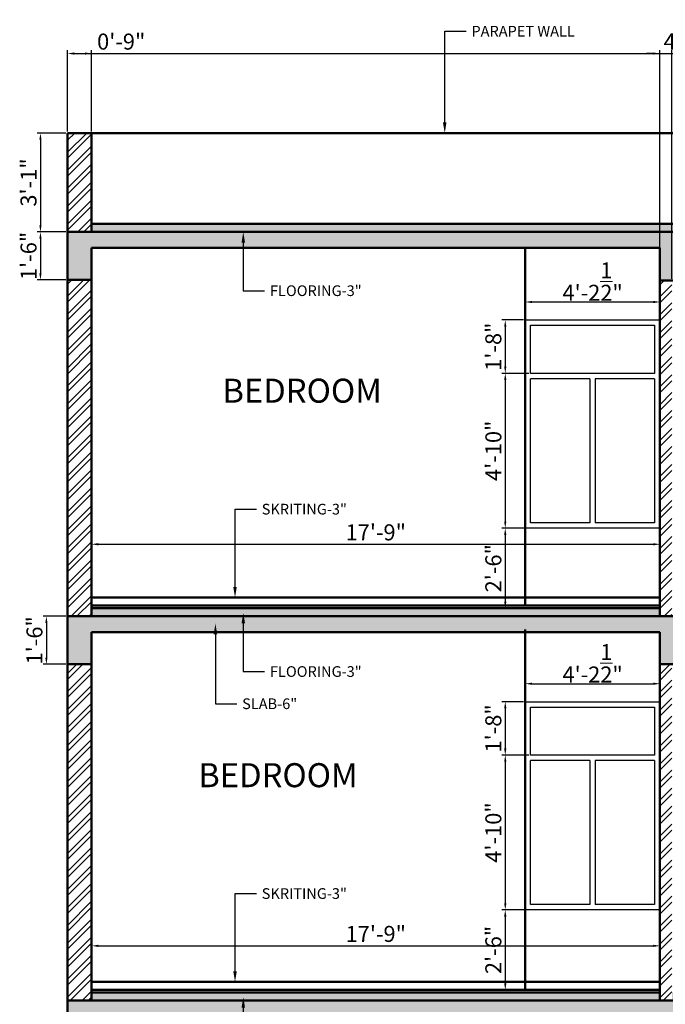
# Model space of a CAD drawing. Units: inches. Extents: x 1615 to 2231, y 1931 to 2519.
# Tile 2 of 6: x 1650 to 1892, y 2150 to 2519. Entities that reach past the tile are written whole.
import ezdxf
from ezdxf import colors
from ezdxf.entities.mleader import LeaderData, LeaderLine
from ezdxf.math import Vec2, Vec3

# ---------------------------------------------------------------- set-up
doc = ezdxf.new("R2010")
doc.units = ezdxf.units.IN
for name, color, linetype, lineweight in [('A-ANNO-DIMS', 2, 'Continuous', 18), ('A-ANNO-NOTE', 3, 'Continuous', 18), ('A-AREA-IDEN', 7, 'Continuous', 25), ('A-GLAZ', 4, 'Continuous', 25), ('A-SECT', 7, 'Continuous', 50), ('A-WALL-PATT', 8, 'Continuous', 13)]:
    doc.layers.add(name, color=color, linetype=linetype, lineweight=lineweight)
doc.styles.get("Standard").update_dxf_attribs({"font": 'arial.ttf'})
doc.dimstyles.new('ISO-25', dxfattribs={"dimtxt": 6, "dimasz": 2.5, "dimexe": 1.25, "dimexo": 0.625, "dimtad": 1, "dimdec": 1, "dimlunit": 4, "dimtxsty": 'Standard', "dimcen": 2.5, "dimadec": 0, "dimazin": 0, "dimtfac": 1, "dimtdec": 1, "dimtmove": 0, "dimatfit": 3, "dimfxl": 1, "dimarcsym": 0})

# ---------------------------------------------------------------- blocks, each defined once
blk = doc.blocks.new('*D2')
at = {"layer": 'A-ANNO-DIMS', "color": 0, "lineweight": -2, "transparency": 16777216}
for p, q in [((1667.24, 2476.53), (1656.46, 2476.53)), ((1657.71, 2474.03), (1657.71, 2442.03)), ((1667.24, 2439.53), (1656.46, 2439.53))]:
    blk.add_line(p, q, dxfattribs=at)
at = {"layer": 'A-ANNO-DIMS', "color": 0, "lineweight": 100, "transparency": 16777216}
for points in [[(1657.29, 2474.03), (1658.12, 2474.03), (1657.71, 2476.53)], [(1657.29, 2442.03), (1658.12, 2442.03), (1657.71, 2439.53)]]:
    blk.add_solid(points, dxfattribs=at)
at = {"layer": 'Defpoints', "color": 0, "lineweight": 100, "transparency": 16777216}
for p in [(1667.87, 2476.53), (1657.71, 2439.53), (1667.87, 2439.53)]:
    blk.add_point(p, dxfattribs=at)
at = {"layer": 'A-ANNO-DIMS', "color": 0, "transparency": 16777216, "insert": (1654.02, 2458.03), "char_height": 6, "attachment_point": 5, "rotation": 90}
blk.add_mtext('3\'-1"', dxfattribs=at)
blk = doc.blocks.new('*D3')
at = {"layer": 'A-ANNO-DIMS', "color": 0, "lineweight": -2, "transparency": 16777216}
for p, q in [((1667.24, 2439.53), (1656.46, 2439.53)), ((1657.71, 2437.03), (1657.71, 2424.03)), ((1667.24, 2421.53), (1656.46, 2421.53))]:
    blk.add_line(p, q, dxfattribs=at)
at = {"layer": 'A-ANNO-DIMS', "color": 0, "lineweight": 100, "transparency": 16777216}
for points in [[(1657.29, 2437.03), (1658.12, 2437.03), (1657.71, 2439.53)], [(1657.29, 2424.03), (1658.12, 2424.03), (1657.71, 2421.53)]]:
    blk.add_solid(points, dxfattribs=at)
at = {"layer": 'Defpoints', "color": 0, "lineweight": 100, "transparency": 16777216}
for p in [(1667.87, 2439.53), (1657.71, 2421.53), (1667.87, 2421.53)]:
    blk.add_point(p, dxfattribs=at)
at = {"layer": 'A-ANNO-DIMS', "color": 0, "transparency": 16777216, "insert": (1654.02, 2430.53), "char_height": 6, "attachment_point": 5, "rotation": 90}
blk.add_mtext('1\'-6"', dxfattribs=at)
blk = doc.blocks.new('*D4')
at = {"layer": 'A-ANNO-DIMS', "color": 0, "lineweight": -2, "transparency": 16777216}
for p, q in [((1667.24, 2295.53), (1658.68, 2295.53)), ((1659.93, 2293.03), (1659.93, 2280.03)), ((1667.24, 2277.53), (1658.68, 2277.53))]:
    blk.add_line(p, q, dxfattribs=at)
at = {"layer": 'A-ANNO-DIMS', "color": 0, "lineweight": 100, "transparency": 16777216}
for points in [[(1659.51, 2293.03), (1660.35, 2293.03), (1659.93, 2295.53)], [(1659.51, 2280.03), (1660.35, 2280.03), (1659.93, 2277.53)]]:
    blk.add_solid(points, dxfattribs=at)
at = {"layer": 'Defpoints', "color": 0, "lineweight": 100, "transparency": 16777216}
for p in [(1667.87, 2295.53), (1659.93, 2277.53), (1667.87, 2277.53)]:
    blk.add_point(p, dxfattribs=at)
at = {"layer": 'A-ANNO-DIMS', "color": 0, "transparency": 16777216, "insert": (1656.24, 2286.53), "char_height": 6, "attachment_point": 5, "rotation": 90}
blk.add_mtext('1\'-6"', dxfattribs=at)
blk = doc.blocks.new('*D33')
at = {"layer": 'A-ANNO-DIMS', "color": 0, "lineweight": -2, "transparency": 16777216}
for p, q in [((1839.37, 2264.15), (1839.37, 2271.52)), ((1841.87, 2270.27), (1887.37, 2270.27)), ((1889.87, 2264.15), (1889.87, 2271.52))]:
    blk.add_line(p, q, dxfattribs=at)
at = {"layer": 'A-ANNO-DIMS', "color": 0, "lineweight": 100, "transparency": 16777216}
for points in [[(1841.87, 2270.68), (1841.87, 2269.85), (1839.37, 2270.27)], [(1887.37, 2270.68), (1887.37, 2269.85), (1889.87, 2270.27)]]:
    blk.add_solid(points, dxfattribs=at)
at = {"layer": 'Defpoints', "color": 0, "lineweight": 100, "transparency": 16777216}
for p in [(1889.87, 2270.27), (1839.37, 2263.53), (1889.87, 2263.53)]:
    blk.add_point(p, dxfattribs=at)
at = {"layer": 'A-ANNO-DIMS', "color": 0, "transparency": 16777216, "insert": (1864.62, 2277.92), "char_height": 6, "attachment_point": 5}
blk.add_mtext('4\'-2{\\H1x;\\S1/2;}"', dxfattribs=at)
blk = doc.blocks.new('*D34')
at = {"layer": 'A-ANNO-DIMS', "color": 0, "lineweight": -2, "transparency": 16777216}
for p, q in [((1838.74, 2263.53), (1830.64, 2263.53)), ((1831.89, 2261.03), (1831.89, 2246.03)), ((1840.74, 2243.53), (1830.64, 2243.53))]:
    blk.add_line(p, q, dxfattribs=at)
at = {"layer": 'A-ANNO-DIMS', "color": 0, "lineweight": 100, "transparency": 16777216}
for points in [[(1831.47, 2261.03), (1832.31, 2261.03), (1831.89, 2263.53)], [(1831.47, 2246.03), (1832.31, 2246.03), (1831.89, 2243.53)]]:
    blk.add_solid(points, dxfattribs=at)
at = {"layer": 'Defpoints', "color": 0, "lineweight": 100, "transparency": 16777216}
for p in [(1839.37, 2263.53), (1831.89, 2243.53), (1841.37, 2243.53)]:
    blk.add_point(p, dxfattribs=at)
at = {"layer": 'A-ANNO-DIMS', "color": 0, "transparency": 16777216, "insert": (1828.2, 2253.53), "char_height": 6, "attachment_point": 5, "rotation": 90}
blk.add_mtext('1\'-8"', dxfattribs=at)
blk = doc.blocks.new('*D35')
at = {"layer": 'A-ANNO-DIMS', "color": 0, "lineweight": -2, "transparency": 16777216}
for p, q in [((1840.74, 2243.53), (1830.64, 2243.53)), ((1831.89, 2241.03), (1831.89, 2188.03)), ((1840.74, 2185.53), (1830.64, 2185.53))]:
    blk.add_line(p, q, dxfattribs=at)
at = {"layer": 'A-ANNO-DIMS', "color": 0, "lineweight": 100, "transparency": 16777216}
for points in [[(1831.47, 2241.03), (1832.31, 2241.03), (1831.89, 2243.53)], [(1831.47, 2188.03), (1832.31, 2188.03), (1831.89, 2185.53)]]:
    blk.add_solid(points, dxfattribs=at)
at = {"layer": 'Defpoints', "color": 0, "lineweight": 100, "transparency": 16777216}
for p in [(1841.37, 2243.53), (1831.89, 2185.53), (1841.37, 2185.53)]:
    blk.add_point(p, dxfattribs=at)
at = {"layer": 'A-ANNO-DIMS', "color": 0, "transparency": 16777216, "insert": (1828.2, 2214.53), "char_height": 6, "attachment_point": 5, "rotation": 90}
blk.add_mtext('4\'-10"', dxfattribs=at)
blk = doc.blocks.new('*D36')
at = {"layer": 'A-ANNO-DIMS', "color": 0, "lineweight": -2, "transparency": 16777216}
for p, q in [((1838.74, 2185.53), (1830.64, 2185.53)), ((1831.89, 2183.03), (1831.89, 2158.03)), ((1838.74, 2155.53), (1830.64, 2155.53))]:
    blk.add_line(p, q, dxfattribs=at)
at = {"layer": 'A-ANNO-DIMS', "color": 0, "lineweight": 100, "transparency": 16777216}
for points in [[(1831.47, 2183.03), (1832.31, 2183.03), (1831.89, 2185.53)], [(1831.47, 2158.03), (1832.31, 2158.03), (1831.89, 2155.53)]]:
    blk.add_solid(points, dxfattribs=at)
at = {"layer": 'Defpoints', "color": 0, "lineweight": 100, "transparency": 16777216}
for p in [(1839.37, 2185.53), (1831.89, 2155.53), (1839.37, 2155.53)]:
    blk.add_point(p, dxfattribs=at)
at = {"layer": 'A-ANNO-DIMS', "color": 0, "transparency": 16777216, "insert": (1828.2, 2170.53), "char_height": 6, "attachment_point": 5, "rotation": 90}
blk.add_mtext('2\'-6"', dxfattribs=at)
blk = doc.blocks.new('*D40')
at = {"layer": 'A-ANNO-DIMS', "color": 0, "lineweight": -2, "transparency": 16777216}
for p, q in [((1839.37, 2407.15), (1839.37, 2414.52)), ((1841.87, 2413.27), (1887.37, 2413.27)), ((1889.87, 2407.15), (1889.87, 2414.52))]:
    blk.add_line(p, q, dxfattribs=at)
at = {"layer": 'A-ANNO-DIMS', "color": 0, "lineweight": 100, "transparency": 16777216}
for points in [[(1841.87, 2413.68), (1841.87, 2412.85), (1839.37, 2413.27)], [(1887.37, 2413.68), (1887.37, 2412.85), (1889.87, 2413.27)]]:
    blk.add_solid(points, dxfattribs=at)
at = {"layer": 'Defpoints', "color": 0, "lineweight": 100, "transparency": 16777216}
for p in [(1889.87, 2413.27), (1839.37, 2406.53), (1889.87, 2406.53)]:
    blk.add_point(p, dxfattribs=at)
at = {"layer": 'A-ANNO-DIMS', "color": 0, "transparency": 16777216, "insert": (1864.62, 2420.92), "char_height": 6, "attachment_point": 5}
blk.add_mtext('4\'-2{\\H1x;\\S1/2;}"', dxfattribs=at)
blk = doc.blocks.new('*D41')
at = {"layer": 'A-ANNO-DIMS', "color": 0, "lineweight": -2, "transparency": 16777216}
for p, q in [((1838.74, 2406.53), (1830.64, 2406.53)), ((1831.89, 2404.03), (1831.89, 2389.03)), ((1840.74, 2386.53), (1830.64, 2386.53))]:
    blk.add_line(p, q, dxfattribs=at)
at = {"layer": 'A-ANNO-DIMS', "color": 0, "lineweight": 100, "transparency": 16777216}
for points in [[(1831.47, 2404.03), (1832.31, 2404.03), (1831.89, 2406.53)], [(1831.47, 2389.03), (1832.31, 2389.03), (1831.89, 2386.53)]]:
    blk.add_solid(points, dxfattribs=at)
at = {"layer": 'Defpoints', "color": 0, "lineweight": 100, "transparency": 16777216}
for p in [(1839.37, 2406.53), (1831.89, 2386.53), (1841.37, 2386.53)]:
    blk.add_point(p, dxfattribs=at)
at = {"layer": 'A-ANNO-DIMS', "color": 0, "transparency": 16777216, "insert": (1828.2, 2396.53), "char_height": 6, "attachment_point": 5, "rotation": 90}
blk.add_mtext('1\'-8"', dxfattribs=at)
blk = doc.blocks.new('*D42')
at = {"layer": 'A-ANNO-DIMS', "color": 0, "lineweight": -2, "transparency": 16777216}
for p, q in [((1840.74, 2386.53), (1830.64, 2386.53)), ((1831.89, 2384.03), (1831.89, 2331.03)), ((1840.74, 2328.53), (1830.64, 2328.53))]:
    blk.add_line(p, q, dxfattribs=at)
at = {"layer": 'A-ANNO-DIMS', "color": 0, "lineweight": 100, "transparency": 16777216}
for points in [[(1831.47, 2384.03), (1832.31, 2384.03), (1831.89, 2386.53)], [(1831.47, 2331.03), (1832.31, 2331.03), (1831.89, 2328.53)]]:
    blk.add_solid(points, dxfattribs=at)
at = {"layer": 'Defpoints', "color": 0, "lineweight": 100, "transparency": 16777216}
for p in [(1841.37, 2386.53), (1831.89, 2328.53), (1841.37, 2328.53)]:
    blk.add_point(p, dxfattribs=at)
at = {"layer": 'A-ANNO-DIMS', "color": 0, "transparency": 16777216, "insert": (1828.2, 2357.53), "char_height": 6, "attachment_point": 5, "rotation": 90}
blk.add_mtext('4\'-10"', dxfattribs=at)
blk = doc.blocks.new('*D43')
at = {"layer": 'A-ANNO-DIMS', "color": 0, "lineweight": -2, "transparency": 16777216}
for p, q in [((1838.74, 2328.53), (1830.64, 2328.53)), ((1831.89, 2326.03), (1831.89, 2301.03)), ((1838.74, 2298.53), (1830.64, 2298.53))]:
    blk.add_line(p, q, dxfattribs=at)
at = {"layer": 'A-ANNO-DIMS', "color": 0, "lineweight": 100, "transparency": 16777216}
for points in [[(1831.47, 2326.03), (1832.31, 2326.03), (1831.89, 2328.53)], [(1831.47, 2301.03), (1832.31, 2301.03), (1831.89, 2298.53)]]:
    blk.add_solid(points, dxfattribs=at)
at = {"layer": 'Defpoints', "color": 0, "lineweight": 100, "transparency": 16777216}
for p in [(1839.37, 2328.53), (1831.89, 2298.53), (1839.37, 2298.53)]:
    blk.add_point(p, dxfattribs=at)
at = {"layer": 'A-ANNO-DIMS', "color": 0, "transparency": 16777216, "insert": (1828.2, 2313.53), "char_height": 6, "attachment_point": 5, "rotation": 90}
blk.add_mtext('2\'-6"', dxfattribs=at)
blk = doc.blocks.new('*D58')
at = {"layer": 'A-ANNO-DIMS', "color": 0, "lineweight": -2, "transparency": 16777216}
for p, q in [((1676.87, 2159.15), (1676.87, 2173.32)), ((1889.87, 2159.15), (1889.87, 2173.32)), ((1679.37, 2172.07), (1887.37, 2172.07))]:
    blk.add_line(p, q, dxfattribs=at)
at = {"layer": 'A-ANNO-DIMS', "color": 0, "lineweight": 100, "transparency": 16777216}
for points in [[(1679.37, 2172.49), (1679.37, 2171.66), (1676.87, 2172.07)], [(1887.37, 2172.49), (1887.37, 2171.66), (1889.87, 2172.07)]]:
    blk.add_solid(points, dxfattribs=at)
at = {"layer": 'Defpoints', "color": 0, "lineweight": 100, "transparency": 16777216}
for p in [(1889.87, 2172.07), (1676.87, 2158.53), (1889.87, 2158.53)]:
    blk.add_point(p, dxfattribs=at)
at = {"layer": 'A-ANNO-DIMS', "color": 0, "transparency": 16777216, "insert": (1783.37, 2175.76), "char_height": 6, "attachment_point": 5}
blk.add_mtext('17\'-9"', dxfattribs=at)
blk = doc.blocks.new('*D59')
at = {"layer": 'A-ANNO-DIMS', "color": 0, "lineweight": -2, "transparency": 16777216}
for p, q in [((1676.87, 2303.15), (1676.87, 2323.76)), ((1679.37, 2322.51), (1887.37, 2322.51)), ((1889.87, 2303.15), (1889.87, 2323.76))]:
    blk.add_line(p, q, dxfattribs=at)
at = {"layer": 'A-ANNO-DIMS', "color": 0, "lineweight": 100, "transparency": 16777216}
for points in [[(1679.37, 2322.93), (1679.37, 2322.09), (1676.87, 2322.51)], [(1887.37, 2322.93), (1887.37, 2322.09), (1889.87, 2322.51)]]:
    blk.add_solid(points, dxfattribs=at)
at = {"layer": 'Defpoints', "color": 0, "lineweight": 100, "transparency": 16777216}
for p in [(1889.87, 2322.51), (1676.87, 2302.53), (1889.87, 2302.53)]:
    blk.add_point(p, dxfattribs=at)
at = {"layer": 'A-ANNO-DIMS', "color": 0, "transparency": 16777216, "insert": (1783.37, 2326.2), "char_height": 6, "attachment_point": 5}
blk.add_mtext('17\'-9"', dxfattribs=at)
blk = doc.blocks.new('WIN-BEDROOM')
for p, q in [((1839.37, 2406.53), (1889.87, 2406.53)), ((1839.37, 2386.53), (1839.37, 2406.53)), ((1889.87, 2406.53), (1889.87, 2386.53)), ((1841.37, 2404.53), (1887.87, 2404.53)), ((1841.37, 2386.53), (1841.37, 2404.53)), ((1887.87, 2404.53), (1887.87, 2386.53)), ((1839.37, 2328.53), (1839.37, 2386.53)), ((1887.87, 2386.53), (1841.37, 2386.53)), ((1841.37, 2330.53), (1841.37, 2384.53)), ((1863.62, 2384.53), (1841.37, 2384.53)), ((1863.62, 2384.53), (1863.62, 2330.53)), ((1887.87, 2384.53), (1865.62, 2384.53)), ((1865.62, 2384.53), (1865.62, 2330.53)), ((1887.87, 2384.53), (1887.87, 2330.53)), ((1889.87, 2386.53), (1889.87, 2328.53)), ((1889.87, 2328.53), (1839.37, 2328.53)), ((1863.62, 2330.53), (1841.37, 2330.53)), ((1887.87, 2330.53), (1865.62, 2330.53))]:
    blk.add_line(p, q)
blk = doc.blocks.new('*D78')
at = {"layer": 'A-ANNO-DIMS', "color": 0, "lineweight": -2, "transparency": 16777216}
for p, q in [((1667.87, 2477.15), (1667.87, 2507.6)), ((1670.37, 2506.35), (2148.87, 2506.35)), ((2151.37, 2477.15), (2151.37, 2507.6))]:
    blk.add_line(p, q, dxfattribs=at)
at = {"layer": 'A-ANNO-DIMS', "color": 0, "lineweight": 100, "transparency": 16777216}
for points in [[(1670.37, 2506.77), (1670.37, 2505.93), (1667.87, 2506.35)], [(2148.87, 2506.77), (2148.87, 2505.93), (2151.37, 2506.35)]]:
    blk.add_solid(points, dxfattribs=at)
at = {"layer": 'Defpoints', "color": 0, "lineweight": 100, "transparency": 16777216}
for p in [(2151.37, 2506.35), (1667.87, 2476.53), (2151.37, 2476.53)]:
    blk.add_point(p, dxfattribs=at)
at = {"layer": 'A-ANNO-DIMS', "color": 0, "transparency": 16777216, "insert": (1909.62, 2510.08), "char_height": 6, "attachment_point": 5}
blk.add_mtext('40\'-3 1/2"', dxfattribs=at)
blk = doc.blocks.new('*D80')
at = {"layer": 'A-ANNO-DIMS', "color": 0, "lineweight": -2, "transparency": 16777216}
for p, q in [((1667.87, 2477.15), (1667.87, 2507.6)), ((1670.37, 2506.35), (1674.37, 2506.35)), ((1676.87, 2477.15), (1676.87, 2507.6)), ((1676.87, 2506.35), (1696.57, 2506.35))]:
    blk.add_line(p, q, dxfattribs=at)
at = {"layer": 'A-ANNO-DIMS', "color": 0, "lineweight": 100, "transparency": 16777216}
for points in [[(1670.37, 2506.77), (1670.37, 2505.93), (1667.87, 2506.35)], [(1674.37, 2506.77), (1674.37, 2505.93), (1676.87, 2506.35)]]:
    blk.add_solid(points, dxfattribs=at)
at = {"layer": 'Defpoints', "color": 0, "lineweight": 100, "transparency": 16777216}
for p in [(1676.87, 2506.35), (1667.87, 2476.53), (1676.87, 2476.53)]:
    blk.add_point(p, dxfattribs=at)
at = {"layer": 'A-ANNO-DIMS', "color": 0, "transparency": 16777216, "insert": (1687.97, 2510.04), "char_height": 6, "attachment_point": 5}
blk.add_mtext('0\'-9"', dxfattribs=at)
blk = doc.blocks.new('*D82')
at = {"layer": 'A-ANNO-DIMS', "color": 0, "lineweight": -2, "transparency": 16777216}
for p, q in [((1887.37, 2506.35), (1884.87, 2506.35)), ((1889.87, 2421.92), (1889.87, 2507.6)), ((1889.87, 2506.35), (1894.37, 2506.35)), ((1894.37, 2421.92), (1894.37, 2507.6)), ((1896.87, 2506.35), (1930.55, 2506.35))]:
    blk.add_line(p, q, dxfattribs=at)
at = {"layer": 'A-ANNO-DIMS', "color": 0, "lineweight": 100, "transparency": 16777216}
for points in [[(1887.37, 2506.77), (1887.37, 2505.93), (1889.87, 2506.35)], [(1896.87, 2506.77), (1896.87, 2505.93), (1894.37, 2506.35)]]:
    blk.add_solid(points, dxfattribs=at)
at = {"layer": 'Defpoints', "color": 0, "lineweight": 100, "transparency": 16777216}
for p in [(1894.37, 2506.35), (1889.87, 2421.29), (1894.37, 2421.29)]:
    blk.add_point(p, dxfattribs=at)
at = {"layer": 'A-ANNO-DIMS', "color": 0, "transparency": 16777216, "insert": (1914.96, 2510.08), "char_height": 6, "attachment_point": 5}
blk.add_mtext('0\'-4 1/2"', dxfattribs=at)

msp = doc.modelspace()

# ---------------------------------------------------------------- hatches: boundary and pattern name
at = {"layer": 'A-WALL-PATT'}
h = msp.add_hatch(dxfattribs=at)
h.set_pattern_fill('ANSI32', color=256, scale=0.5)
h.paths.add_polyline_path([(1676.87, 2421.53), (1667.87, 2421.53), (1667.87, 2295.53), (1676.87, 2295.53)])
h.paths.add_polyline_path([(1676.87, 2277.53), (1667.87, 2277.53), (1667.87, 2151.53), (1676.87, 2151.53)])
h.paths.add_polyline_path([(1676.87, 2476.53), (1667.87, 2476.53), (1667.87, 2439.53), (1676.87, 2439.53)])
h.paths.add_polyline_path([(1894.37, 2421.29), (1889.87, 2421.29), (1889.87, 2295.53), (1894.37, 2295.53)])
h.paths.add_polyline_path([(1974.87, 2421.29), (1965.87, 2421.29), (1965.87, 2295.53), (1974.87, 2295.53)])
h.paths.add_polyline_path([(2151.37, 2421.29), (2142.37, 2421.29), (2142.37, 2295.53), (2151.37, 2295.53)])
h.paths.add_polyline_path([(2151.37, 2476.53), (2142.37, 2476.53), (2142.37, 2442.53), (2151.37, 2442.53)])
h.paths.add_polyline_path([(1974.87, 2277.53), (1965.87, 2277.53), (1965.87, 2151.53), (1974.87, 2151.53)])
h.paths.add_polyline_path([(1974.87, 2133.53), (1965.87, 2133.53), (1965.87, 2060.03), (1974.87, 2060.03)])
h.paths.add_polyline_path([(2098.87, 2145.53), (2094.37, 2145.53), (2094.37, 2059.03), (2098.87, 2059.03)])
h = msp.add_hatch(dxfattribs=at)
h.set_pattern_fill('DOTS', color=256, scale=0.5)
h.paths.add_polyline_path([(2142.37, 2442.53), (1839.37, 2442.53), (1676.87, 2442.53), (1676.87, 2439.53), (2142.37, 2439.53)])
h.paths.add_polyline_path([(1889.87, 2298.53), (1676.87, 2298.53), (1676.87, 2295.53), (1889.87, 2295.53)])
h.paths.add_polyline_path([(2142.37, 2298.53), (1974.87, 2298.53), (1974.87, 2295.53), (2142.37, 2295.53)])
h.paths.add_polyline_path([(1889.87, 2154.53), (1676.87, 2154.53), (1676.87, 2151.53), (1889.87, 2151.53)])
h.paths.add_polyline_path([(1965.87, 2154.53), (1894.37, 2154.53), (1894.37, 2151.53), (1965.87, 2151.53)])
h.paths.add_polyline_path([(2142.37, 2154.53), (1974.87, 2154.53), (1974.87, 2151.53), (2142.37, 2151.53)])
h.paths.add_polyline_path([(2094.37, 2062.03), (1974.87, 2062.03), (1974.87, 2059.03), (2094.37, 2059.03)])
h.paths.add_polyline_path([(2142.37, 2062.03), (2098.87, 2062.03), (2098.87, 2059.03), (2142.37, 2059.03)])
h.paths.add_polyline_path([(1956.87, 2049.53), (1693.37, 2049.53), (1693.37, 2046.53), (1956.87, 2046.53)])
h = msp.add_hatch(dxfattribs=at)
h.set_pattern_fill('AR-CONC', color=256, scale=0.1)
h.paths.add_polyline_path([(1898.87, 2151.53), (1667.87, 2151.53), (1667.87, 2145.53), (1679.87, 2145.53), (1682.87, 2145.53), (1889.87, 2145.53), (1889.87, 2133.53), (1974.87, 2133.53), (1974.87, 2145.53), (2142.37, 2145.53), (2142.37, 2133.53), (2157.37, 2133.53), (2157.37, 2151.53), (2155.87, 2151.53), (2151.37, 2151.53), (1965.87, 2151.53), (1965.87, 2139.53), (1898.87, 2139.53)])
h.paths.add_polyline_path([(1898.87, 2295.53), (1667.87, 2295.53), (1667.87, 2277.53), (1676.87, 2277.53), (1676.87, 2289.53), (1889.87, 2289.53), (1889.87, 2277.53), (1974.87, 2277.53), (1974.87, 2289.53), (2142.37, 2289.53), (2142.37, 2277.53), (2151.37, 2277.53), (2151.37, 2295.53), (1965.87, 2295.53), (1965.87, 2283.53), (1898.87, 2283.53)])
h.paths.add_polyline_path([(2142.37, 2439.53), (1676.87, 2439.53), (1667.87, 2439.53), (1667.87, 2421.53), (1676.87, 2421.53), (1676.87, 2433.53), (1889.87, 2433.53), (1889.87, 2421.29), (1898.87, 2421.29), (1898.87, 2433.53), (1965.87, 2433.53), (1965.87, 2421.29), (1974.87, 2421.29), (1974.87, 2433.53), (2142.37, 2433.53)])
h = msp.add_hatch(dxfattribs=at)
h.set_pattern_fill('ANSI32', color=256, scale=0.5)
h.paths.add_polyline_path([(2151.37, 2277.53), (2142.37, 2277.53), (2142.37, 2151.53), (2151.37, 2151.53)])
h.paths.add_polyline_path([(1894.37, 2277.53), (1889.87, 2277.53), (1889.87, 2151.53), (1894.37, 2151.53)])

# ---------------------------------------------------------------- linework, layer by layer
at = {"layer": 'A-SECT'}
for p, q in [((1667.87, 2476.53), (1667.87, 2145.53)), ((1667.87, 2476.53), (2151.37, 2476.53)), ((1676.87, 2476.53), (1676.87, 2439.53)), ((1676.87, 2442.53), (1889.87, 2442.53)), ((1839.37, 2442.53), (2151.37, 2442.53)), ((1667.87, 2439.53), (1889.87, 2439.53)), ((1676.87, 2439.53), (2142.37, 2439.53)), ((1676.87, 2433.53), (1889.87, 2433.53)), ((1676.87, 2433.53), (1676.87, 2295.53)), ((1839.37, 2433.53), (1839.37, 2299.53)), ((1889.87, 2433.53), (1889.87, 2295.53)), ((1667.87, 2421.53), (1676.87, 2421.53)), ((1889.87, 2421.29), (1898.87, 2421.29)), ((1676.87, 2302.53), (1889.87, 2302.53)), ((1676.87, 2299.53), (1889.87, 2299.53)), ((1676.87, 2298.53), (1889.87, 2298.53)), ((1667.87, 2295.53), (2151.37, 2295.53)), ((1676.87, 2289.53), (1889.87, 2289.53)), ((1676.87, 2289.53), (1676.87, 2151.53)), ((1839.37, 2290.53), (1839.37, 2155.53)), ((1889.87, 2289.53), (1889.87, 2151.53)), ((1667.87, 2277.53), (1676.87, 2277.53)), ((1889.87, 2277.53), (1974.87, 2277.53)), ((1676.87, 2158.53), (1889.87, 2158.53)), ((1676.87, 2155.53), (1889.87, 2155.53)), ((1676.87, 2154.53), (1889.87, 2154.53)), ((1667.87, 2151.53), (2151.37, 2151.53))]:
    msp.add_line(p, q, dxfattribs=at)

# ---------------------------------------------------------------- block references
at = {"layer": 'A-GLAZ'}
for p in [(0, 0), (0, -143)]:
    msp.add_blockref('WIN-BEDROOM', p, dxfattribs=at)

# ---------------------------------------------------------------- texts
at = {"layer": 'A-AREA-IDEN', "char_height": 9, "attachment_point": 1}
for insert in [(1725.9, 2384.54), (1716.84, 2240.5)]:
    msp.add_mtext_dynamic_manual_height_columns('BEDROOM', width=2.6039, gutter_width=12.5, heights=[0], dxfattribs=dict(at, insert=insert))

# ---------------------------------------------------------------- dimensions: what is measured, and where the dimension line sits
at = {"layer": 'A-ANNO-DIMS'}
for base, p1, p2, override, picture, middle in [((2151.37, 2506.35), (1667.87, 2476.53), (2151.37, 2476.53), {"dimdec": 1, "dimlfac": 1, "dimrnd": 0, "dimzin": 1, "dimdsep": 46, "dimlunit": 4, "dimfrac": 2}, '*D78', (1909.62, 2510.08)), ((1894.37, 2506.35), (1889.87, 2421.29), (1894.37, 2421.29), {"dimdec": 1, "dimlfac": 1, "dimrnd": 0, "dimzin": 1, "dimdsep": 46, "dimlunit": 4, "dimfrac": 2}, '*D82', (1914.96, 2510.08)), ((1676.87, 2506.35), (1667.87, 2476.53), (1676.87, 2476.53), {"dimdec": 1, "dimlfac": 1, "dimrnd": 0, "dimzin": 1, "dimdsep": 46, "dimlunit": 4, "dimfrac": 2}, '*D80', (1687.97, 2510.04)), ((1889.87, 2413.27), (1839.37, 2406.53), (1889.87, 2406.53), {"dimclrd": 0, "dimclre": 0, "dimclrt": 0}, '*D40', (1864.62, 2420.92)), ((1889.87, 2322.51), (1676.87, 2302.53), (1889.87, 2302.53), {"dimclrd": 0, "dimclre": 0, "dimclrt": 0}, '*D59', (1783.37, 2326.2)), ((1889.87, 2270.27), (1839.37, 2263.53), (1889.87, 2263.53), {"dimclrd": 0, "dimclre": 0, "dimclrt": 0}, '*D33', (1864.62, 2277.92)), ((1889.87, 2172.07), (1676.87, 2158.53), (1889.87, 2158.53), {"dimclrd": 0, "dimclre": 0, "dimclrt": 0}, '*D58', (1783.37, 2175.76))]:
    dim = msp.add_linear_dim(base=base, p1=p1, p2=p2, dimstyle='ISO-25', override=override, dxfattribs=at)
    dim.commit()
    dim.dimension.update_dxf_attribs({"geometry": picture, "text_midpoint": middle})
for base, p1, p2, picture, middle in [((1657.71, 2439.53), (1667.87, 2476.53), (1667.87, 2439.53), '*D2', (1654.02, 2458.03)), ((1657.71, 2421.53), (1667.87, 2439.53), (1667.87, 2421.53), '*D3', (1654.02, 2430.53)), ((1831.89, 2386.53), (1839.37, 2406.53), (1841.37, 2386.53), '*D41', (1828.2, 2396.53)), ((1831.89, 2328.53), (1841.37, 2386.53), (1841.37, 2328.53), '*D42', (1828.2, 2357.53)), ((1831.89, 2298.53), (1839.37, 2328.53), (1839.37, 2298.53), '*D43', (1828.2, 2313.53)), ((1659.93, 2277.53), (1667.87, 2295.53), (1667.87, 2277.53), '*D4', (1656.24, 2286.53)), ((1831.89, 2243.53), (1839.37, 2263.53), (1841.37, 2243.53), '*D34', (1828.2, 2253.53)), ((1831.89, 2185.53), (1841.37, 2243.53), (1841.37, 2185.53), '*D35', (1828.2, 2214.53)), ((1831.89, 2155.53), (1839.37, 2185.53), (1839.37, 2155.53), '*D36', (1828.2, 2170.53))]:
    dim = msp.add_linear_dim(base=base, p1=p1, p2=p2, angle=90, dimstyle='ISO-25', override={"dimclrd": 0, "dimclre": 0, "dimclrt": 0}, dxfattribs=at)
    dim.commit()
    dim.dimension.update_dxf_attribs({"geometry": picture, "text_midpoint": middle})

# ---------------------------------------------------------------- leaders
at = {"layer": 'A-ANNO-NOTE'}
ml = msp.add_multileader_mtext('Standard', dxfattribs=at)
ml.set_content('PARAPET WALL', color=256)
ml.set_leader_properties()
ml.build(insert=Vec2(0, 0))
ctx = ml.context
ctx.base_point, ctx.plane_origin = Vec3(1817.21, 2514.72), Vec3(1809.21, 2476.53)
notes = []
notes.append((ctx, [(0, (1, 1, 0), (1809.21, 2514.72), (1, 0), 8, [(0, [(1809.21, 2476.53)], 0, [])])]))
ctx.mtext.insert, ctx.mtext.flow_direction = Vec3(1819.21, 2516.72), 5
ml = msp.add_multileader_mtext('Standard', dxfattribs=at)
ml.set_content('FLOORING-3"', color=256)
ml.set_leader_properties()
ml.build(insert=Vec2(0, 0))
ctx = ml.context
ctx.base_point, ctx.plane_origin = Vec3(1741.72, 2417.47), Vec3(1733.72, 2439.53)
notes.append((ctx, [(0, (1, 1, 0), (1733.72, 2417.47), (1, 0), 8, [(0, [(1733.72, 2439.53)], 0, [])])]))
ctx.mtext.insert, ctx.mtext.flow_direction = Vec3(1743.72, 2419.5), 5
ml = msp.add_multileader_mtext('Standard', dxfattribs=at)
ml.set_content('SKRITING-3"', color=256)
ml.set_leader_properties()
ml.build(insert=Vec2(0, 0))
ctx = ml.context
ctx.base_point, ctx.plane_origin = Vec3(1738.62, 2335.63), Vec3(1730.62, 2302.53)
notes.append((ctx, [(0, (1, 1, 0), (1730.62, 2335.63), (1, 0), 8, [(0, [(1730.62, 2302.53)], 0, [])])]))
ctx.mtext.insert, ctx.mtext.flow_direction = Vec3(1740.62, 2337.66), 5
ml = msp.add_multileader_mtext('Standard', dxfattribs=at)
ml.set_content('FLOORING-3"', color=256)
ml.set_leader_properties()
ml.build(insert=Vec2(0, 0))
ctx = ml.context
ctx.base_point, ctx.plane_origin = Vec3(1741.72, 2274.79), Vec3(1733.72, 2296.85)
notes.append((ctx, [(0, (1, 1, 0), (1733.72, 2274.79), (1, 0), 8, [(0, [(1733.72, 2296.85)], 0, [])])]))
ctx.mtext.insert, ctx.mtext.flow_direction = Vec3(1743.72, 2276.83), 5
ml = msp.add_multileader_mtext('Standard', dxfattribs=at)
ml.set_content('SLAB-6"', color=256)
ml.set_leader_properties()
ml.build(insert=Vec2(0, 0))
ctx = ml.context
ctx.base_point, ctx.plane_origin = Vec3(1731.29, 2262.73), Vec3(1723.29, 2292.8)
notes.append((ctx, [(0, (1, 1, 0), (1723.29, 2262.73), (1, 0), 8, [(0, [(1723.29, 2292.8)], 0, [])])]))
ctx.mtext.insert, ctx.mtext.flow_direction = Vec3(1733.29, 2264.76), 5
ml = msp.add_multileader_mtext('Standard', dxfattribs=at)
ml.set_content('SKRITING-3"', color=256)
ml.set_leader_properties()
ml.build(insert=Vec2(0, 0))
ctx = ml.context
ctx.base_point, ctx.plane_origin = Vec3(1738.62, 2191.63), Vec3(1730.62, 2158.53)
notes.append((ctx, [(0, (1, 1, 0), (1730.62, 2191.63), (1, 0), 8, [(0, [(1730.62, 2158.53)], 0, [])])]))
ctx.mtext.insert, ctx.mtext.flow_direction = Vec3(1740.62, 2193.66), 5
ml = msp.add_multileader_mtext('Standard', dxfattribs=at)
ml.set_content('FLOORING-3"', color=256)
ml.set_leader_properties()
ml.build(insert=Vec2(0, 0))
ctx = ml.context
ctx.base_point, ctx.plane_origin = Vec3(1741.72, 2130.79), Vec3(1733.72, 2152.85)
notes.append((ctx, [(0, (1, 1, 0), (1733.72, 2130.79), (1, 0), 8, [(0, [(1733.72, 2152.85)], 0, [])])]))
ctx.mtext.insert, ctx.mtext.flow_direction = Vec3(1743.72, 2132.83), 5
for ctx, leaders in notes:
    for number, flags, end, landing, length, lines in leaders:
        leader = LeaderData()
        leader.index, (leader.has_last_leader_line, leader.has_dogleg_vector, leader.attachment_direction) = number, flags
        leader.last_leader_point, leader.dogleg_vector, leader.dogleg_length = Vec3(end), Vec3(landing), length
        for number, points, colour, breaks in lines:
            line = LeaderLine()
            line.index, line.vertices, line.color, line.breaks = number, Vec3.list(points), colors.encode_raw_color(colour), breaks
            leader.lines.append(line)
        ctx.leaders.append(leader)

doc.saveas('drawing.dxf')
